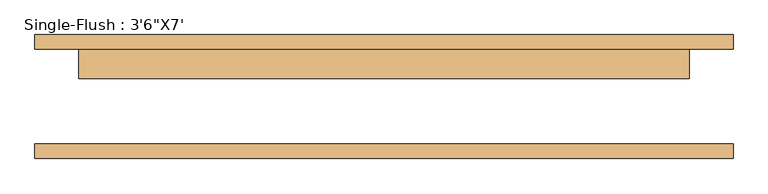
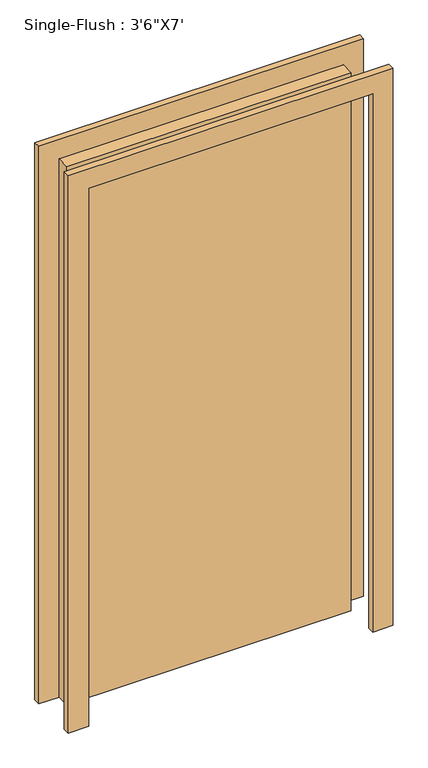
"""IFC4 building model written with IfcOpenShell, lengths in millimetres: door geometry."""

from ifc_helpers import new_model, si_unit, frame, origin, origin_with_axes, place, context, project, spatial, polyline, outline, extrude, source, transform, mapped, element, save


def door_11d56761(model_context):
    return source(origin(), model_context, "Body", "SweptSolid", [
        extrude(outline(polyline([(2209.8, -609.6), (0.0, -609.6), (0.0, -533.4), (2133.6, -533.4), (2133.6, 533.4), (0.0, 533.4), (0.0, 609.6), (2209.8, 609.6), (2209.8, -609.6)])), frame((0.0, 82.9, 0.0), z_axis=(0.0, 1.0, 0.0), x_axis=(0.0, 0.0, 1.0)), (0.0, 0.0, 1.0), 25.4),
        extrude(outline(polyline([(2209.8, 609.6), (2209.8, -609.6), (0.0, -609.6), (0.0, -533.4), (2133.6, -533.4), (2133.6, 533.4), (0.0, 533.4), (0.0, 609.6), (2209.8, 609.6)])), frame((0.0, -108.3, 0.0), z_axis=(0.0, 1.0, 0.0), x_axis=(0.0, 0.0, 1.0)), (0.0, 0.0, 1.0), 25.4),
        extrude(outline(polyline([(533.4, 32.1), (-533.4, 32.1), (-533.4, 82.9), (533.4, 82.9), (533.4, 32.1)])), origin_with_axes(), (0.0, 0.0, 1.0), 2133.6),
    ])


if __name__ == "__main__":
    model = new_model("IFC4")
    model_context = context("Model", 3, world=origin())
    ifc_project = project(units=[si_unit("LENGTHUNIT", "METRE", prefix="MILLI")], contexts=[model_context])
    site = spatial("IfcSite", under=ifc_project)
    building = spatial("IfcBuilding", under=site)
    placement = place(None, origin())
    door_shape = door_11d56761(model_context)
    element("IfcDoor", 1, ObjectType="Single-Flush : 3'6\"X7'", at=placement, inside=building, context=model_context, shape_type="MappedRepresentation", body=[
        mapped(door_shape, transform((0.0, 0.0, 0.0), x_axis=(1.0, 0.0, 0.0), y_axis=(0.0, 1.0, 0.0), z_axis=(0.0, 0.0, 1.0))),
    ])
    save(model, "model.ifc")

# Revit data of these elements
# Type "Single-Flush : 3'6\"X7'"
#   Type Mark = "8"
#   Assembly Code = "C1020"
#   Thickness = 0' - 2"
#   Height = 7' - 0"
#   Trim Projection Ext = 0' - 1"
#   Trim Projection Int = 0' - 1"
#   Trim Width = 0' - 3"
#   Width = 3' - 6"
#   Door Material = Door - Panel
#   Frame Material = Door - Frame
#   Function = (empty or 0)
#   Wall Closure = (empty or 0)
# Element 1 (IfcDoor, "Single-Flush : 3'6\"X7'")
#   Materials on its faces: "Door - Frame", "Door - Panel"
# Materials
#   "Door - Panel": class "Wood", colour RGB 114 82 51, transparency 0
#   "Door - Frame": colour RGB 153 76 43, transparency 0
